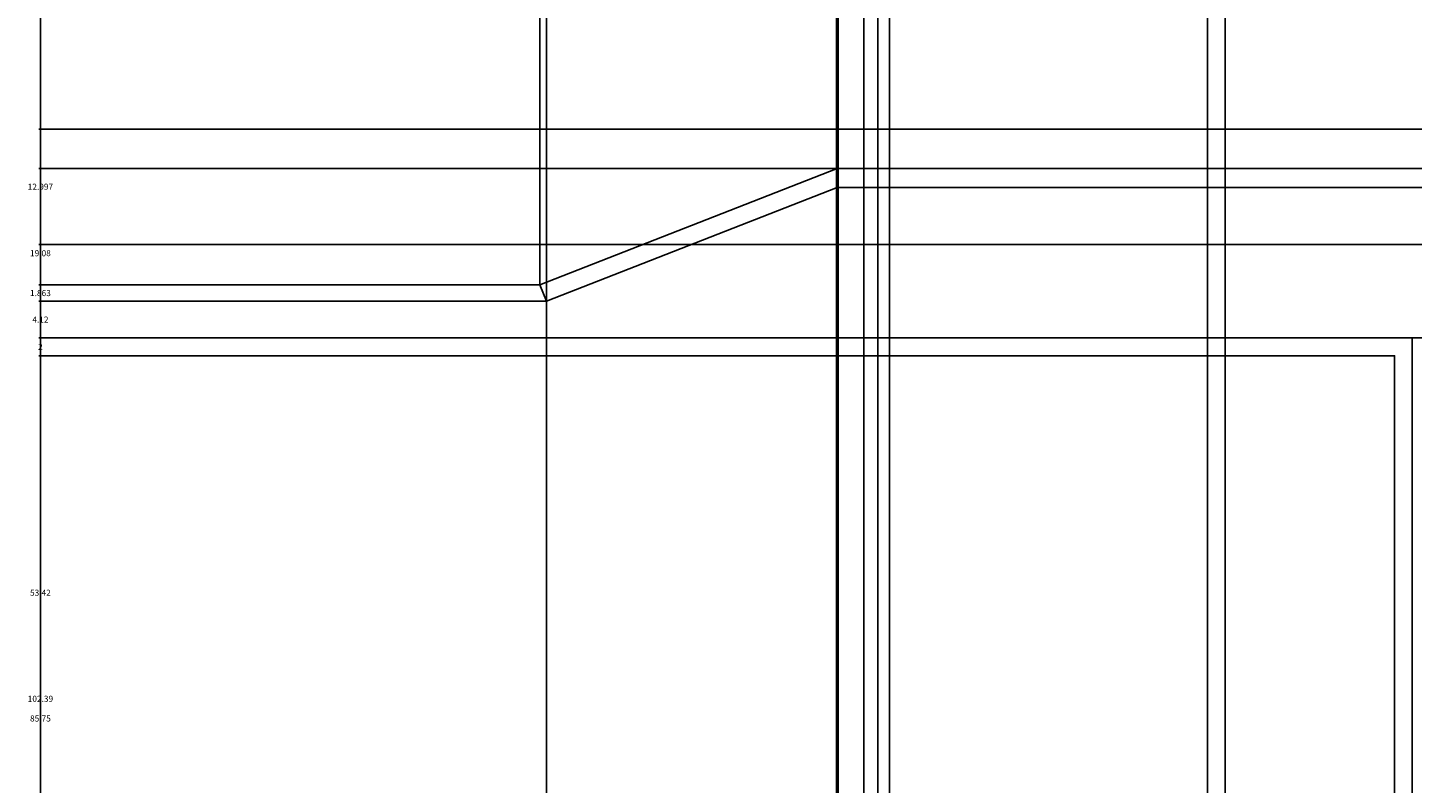
# Model space of a CAD drawing. Units: inches. Extents: x -139 to 346, y 72 to 413.
# Tile 2 of 18: x -139 to 18, y 157 to 242. Entities that reach past the tile are written whole.
import ezdxf

# ---------------------------------------------------------------- set-up
doc = ezdxf.new("R2010")
doc.units = ezdxf.units.IN
doc.header["$MEASUREMENT"] = 0
for name, color, linetype, lineweight in [('A-ANNO-DIMS', 2, 'Continuous', 18), ('A-ELEV', 9, 'Continuous', 25), ('A-GLAZ', 4, 'Continuous', 25), ('A-WALL', 7, 'Continuous', 50)]:
    doc.layers.add(name, color=color, linetype=linetype, lineweight=lineweight)
doc.styles.get("Standard").update_dxf_attribs({"font": 'arial.ttf'})
doc.dimstyles.get("Standard").update_dxf_attribs({"dimtxt": 0.6875, "dimasz": 0.18, "dimexe": 0.18, "dimexo": 0.0625, "dimgap": 0.09, "dimtad": 0, "dimtih": 1, "dimtoh": 1, "dimdec": 4, "dimzin": 0, "dimdsep": 46, "dimlunit": 4, "dimtxsty": 'Standard', "dimcen": 0.09, "dimadec": 0, "dimazin": 0, "dimtfac": 1, "dimtdec": 4, "dimtofl": 0, "dimtmove": 0, "dimatfit": 3, "dimfxl": 1, "dimtolj": 1, "dimtzin": 0, "dimarcsym": 0})

# ---------------------------------------------------------------- blocks, each defined once
blk = doc.blocks.new('*D41')
at = {"layer": 'A-ANNO-DIMS', "color": 0, "lineweight": -2, "transparency": 16777216}
for p, q in [((-47.34, 207.52), (-137.3, 207.52)), ((-137.12, 207.34), (-137.12, 165.09)), ((-137.12, 121.96), (-137.12, 164.21)), ((-5.6, 121.78), (-137.3, 121.78))]:
    blk.add_line(p, q, dxfattribs=at)
at = {"layer": 'A-ANNO-DIMS', "color": 0, "transparency": 16777216}
for points in [[(-137.15, 207.34), (-137.09, 207.34), (-137.12, 207.52)], [(-137.15, 121.96), (-137.09, 121.96), (-137.12, 121.78)]]:
    blk.add_solid(points, dxfattribs=at)
at = {"layer": 'Defpoints', "color": 0, "transparency": 16777216}
for p in [(-137.12, 207.52), (-47.27, 207.52), (-5.54, 121.78)]:
    blk.add_point(p, dxfattribs=at)
at = {"layer": 'A-ANNO-DIMS', "color": 0, "transparency": 16777216, "insert": (-137.12, 164.65), "char_height": 0.688, "attachment_point": 5}
blk.add_mtext('\\A1;85.75', dxfattribs=at)
blk = doc.blocks.new('*D42')
at = {"layer": 'A-ANNO-DIMS', "color": 0, "lineweight": -2, "transparency": 16777216}
for p, q in [((-47.34, 289.06), (-137.3, 289.06)), ((-137.12, 288.88), (-137.12, 248.73)), ((-137.12, 207.7), (-137.12, 247.85)), ((-47.34, 207.52), (-137.3, 207.52))]:
    blk.add_line(p, q, dxfattribs=at)
at = {"layer": 'A-ANNO-DIMS', "color": 0, "transparency": 16777216}
for points in [[(-137.15, 288.88), (-137.09, 288.88), (-137.12, 289.06)], [(-137.15, 207.7), (-137.09, 207.7), (-137.12, 207.52)]]:
    blk.add_solid(points, dxfattribs=at)
at = {"layer": 'Defpoints', "color": 0, "transparency": 16777216}
for p in [(-137.12, 289.06), (-47.27, 289.06), (-47.27, 207.52)]:
    blk.add_point(p, dxfattribs=at)
at = {"layer": 'A-ANNO-DIMS', "color": 0, "transparency": 16777216, "insert": (-137.12, 248.29), "char_height": 0.688, "attachment_point": 5}
blk.add_mtext('\\A1;81.54', dxfattribs=at)
blk = doc.blocks.new('*D48')
at = {"layer": 'A-ANNO-DIMS', "color": 0, "lineweight": -2, "transparency": 16777216}
for p, q in [((-47.34, 226.61), (-137.3, 226.61)), ((-137.12, 226.43), (-137.12, 217.51)), ((-137.12, 207.7), (-137.12, 216.62)), ((-47.34, 207.52), (-137.3, 207.52))]:
    blk.add_line(p, q, dxfattribs=at)
at = {"layer": 'A-ANNO-DIMS', "color": 0, "transparency": 16777216}
for points in [[(-137.15, 226.43), (-137.09, 226.43), (-137.12, 226.61)], [(-137.15, 207.7), (-137.09, 207.7), (-137.12, 207.52)]]:
    blk.add_solid(points, dxfattribs=at)
at = {"layer": 'Defpoints', "color": 0, "transparency": 16777216}
for p in [(-137.12, 226.61), (-47.27, 226.61), (-47.27, 207.52)]:
    blk.add_point(p, dxfattribs=at)
at = {"layer": 'A-ANNO-DIMS', "color": 0, "transparency": 16777216, "insert": (-137.12, 217.07), "char_height": 0.688, "attachment_point": 5}
blk.add_mtext('\\A1;19.08', dxfattribs=at)
blk = doc.blocks.new('*D49')
at = {"layer": 'A-ANNO-DIMS', "color": 0, "lineweight": -2, "transparency": 16777216}
for p, q in [((-80.8, 213.57), (-80.8, 412.45)), ((-80.62, 412.27), (-65.28, 412.27)), ((-47.45, 412.27), (-62.79, 412.27)), ((-47.27, 226.67), (-47.27, 412.45))]:
    blk.add_line(p, q, dxfattribs=at)
at = {"layer": 'A-ANNO-DIMS', "color": 0, "transparency": 16777216}
for points in [[(-80.62, 412.3), (-80.62, 412.24), (-80.8, 412.27)], [(-47.45, 412.3), (-47.45, 412.24), (-47.27, 412.27)]]:
    blk.add_solid(points, dxfattribs=at)
at = {"layer": 'Defpoints', "color": 0, "transparency": 16777216}
for p in [(-47.27, 412.27), (-47.27, 226.61), (-80.8, 213.51)]:
    blk.add_point(p, dxfattribs=at)
at = {"layer": 'A-ANNO-DIMS', "color": 0, "transparency": 16777216, "insert": (-64.03, 412.27), "char_height": 0.688, "attachment_point": 5}
blk.add_mtext('\\A1;33.52', dxfattribs=at)
blk = doc.blocks.new('*D50')
at = {"layer": 'A-ANNO-DIMS', "color": 0, "lineweight": -2, "transparency": 16777216}
for p, q in [((-80.8, 213.57), (-80.8, 412.45)), ((-80.62, 412.27), (-80.25, 412.27)), ((-80.07, 211.71), (-80.07, 412.45)), ((-80.07, 412.27), (-79.89, 412.27))]:
    blk.add_line(p, q, dxfattribs=at)
at = {"layer": 'A-ANNO-DIMS', "color": 0, "transparency": 16777216}
for points in [[(-80.62, 412.3), (-80.62, 412.24), (-80.8, 412.27)], [(-80.25, 412.3), (-80.25, 412.24), (-80.07, 412.27)]]:
    blk.add_solid(points, dxfattribs=at)
at = {"layer": 'Defpoints', "color": 0, "transparency": 16777216}
for p in [(-80.07, 412.27), (-80.8, 213.51), (-80.07, 211.65)]:
    blk.add_point(p, dxfattribs=at)
at = {"layer": 'A-ANNO-DIMS', "color": 0, "transparency": 16777216, "insert": (-78.91, 412.27), "char_height": 0.688, "attachment_point": 5}
blk.add_mtext('\\A1;0.73', dxfattribs=at)
blk = doc.blocks.new('*D51')
at = {"layer": 'A-ANNO-DIMS', "color": 0, "lineweight": -2, "transparency": 16777216}
for p, q in [((-80.07, 207.46), (-80.07, 72.49)), ((-47.27, 207.46), (-47.27, 72.49)), ((-79.89, 72.67), (-65.19, 72.67)), ((-47.45, 72.67), (-62.15, 72.67))]:
    blk.add_line(p, q, dxfattribs=at)
at = {"layer": 'A-ANNO-DIMS', "color": 0, "transparency": 16777216}
for points in [[(-79.89, 72.7), (-79.89, 72.64), (-80.07, 72.67)], [(-47.45, 72.7), (-47.45, 72.64), (-47.27, 72.67)]]:
    blk.add_solid(points, dxfattribs=at)
at = {"layer": 'Defpoints', "color": 0, "transparency": 16777216}
for p in [(-80.07, 207.52), (-47.27, 207.52), (-47.27, 72.67)]:
    blk.add_point(p, dxfattribs=at)
at = {"layer": 'A-ANNO-DIMS', "color": 0, "transparency": 16777216, "insert": (-63.67, 72.67), "char_height": 0.688, "attachment_point": 5}
blk.add_mtext('\\A1;32.795', dxfattribs=at)
blk = doc.blocks.new('*D52')
at = {"layer": 'A-ANNO-DIMS', "color": 0, "lineweight": -2, "transparency": 16777216}
for p, q in [((-80.13, 211.65), (-137.3, 211.65)), ((-137.12, 211.47), (-137.12, 210.02)), ((-137.12, 207.7), (-137.12, 209.15)), ((-80.13, 207.52), (-137.3, 207.52))]:
    blk.add_line(p, q, dxfattribs=at)
at = {"layer": 'A-ANNO-DIMS', "color": 0, "transparency": 16777216}
for points in [[(-137.15, 211.47), (-137.09, 211.47), (-137.12, 211.65)], [(-137.15, 207.7), (-137.09, 207.7), (-137.12, 207.52)]]:
    blk.add_solid(points, dxfattribs=at)
at = {"layer": 'Defpoints', "color": 0, "transparency": 16777216}
for p in [(-137.12, 211.65), (-80.07, 211.65), (-80.07, 207.52)]:
    blk.add_point(p, dxfattribs=at)
at = {"layer": 'A-ANNO-DIMS', "color": 0, "transparency": 16777216, "insert": (-137.12, 209.59), "char_height": 0.688, "attachment_point": 5}
blk.add_mtext('\\A1;4.12', dxfattribs=at)
blk = doc.blocks.new('*D53')
at = {"layer": 'A-ANNO-DIMS', "color": 0, "lineweight": -2, "transparency": 16777216}
for p, q in [((-80.86, 213.51), (-137.3, 213.51)), ((-137.12, 213.33), (-137.12, 213.02)), ((-80.13, 211.65), (-137.3, 211.65)), ((-137.12, 211.83), (-137.12, 212.14))]:
    blk.add_line(p, q, dxfattribs=at)
at = {"layer": 'A-ANNO-DIMS', "color": 0, "transparency": 16777216}
for points in [[(-137.15, 213.33), (-137.09, 213.33), (-137.12, 213.51)], [(-137.15, 211.83), (-137.09, 211.83), (-137.12, 211.65)]]:
    blk.add_solid(points, dxfattribs=at)
at = {"layer": 'Defpoints', "color": 0, "transparency": 16777216}
for p in [(-137.12, 213.51), (-80.8, 213.51), (-80.07, 211.65)]:
    blk.add_point(p, dxfattribs=at)
at = {"layer": 'A-ANNO-DIMS', "color": 0, "transparency": 16777216, "insert": (-137.12, 212.58), "char_height": 0.688, "attachment_point": 5}
blk.add_mtext('\\A1;1.863', dxfattribs=at)
blk = doc.blocks.new('*D54')
at = {"layer": 'A-ANNO-DIMS', "color": 0, "lineweight": -2, "transparency": 16777216}
for p, q in [((-47.21, 224.46), (344.39, 224.46)), ((344.21, 224.28), (344.21, 216.43)), ((344.21, 207.7), (344.21, 215.55)), ((-47.21, 207.52), (344.39, 207.52))]:
    blk.add_line(p, q, dxfattribs=at)
at = {"layer": 'A-ANNO-DIMS', "color": 0, "transparency": 16777216}
for points in [[(344.18, 224.28), (344.24, 224.28), (344.21, 224.46)], [(344.18, 207.7), (344.24, 207.7), (344.21, 207.52)]]:
    blk.add_solid(points, dxfattribs=at)
at = {"layer": 'Defpoints', "color": 0, "transparency": 16777216}
for p in [(-47.27, 224.46), (344.21, 224.46), (-47.27, 207.52)]:
    blk.add_point(p, dxfattribs=at)
at = {"layer": 'A-ANNO-DIMS', "color": 0, "transparency": 16777216, "insert": (344.21, 215.99), "char_height": 0.688, "attachment_point": 5}
blk.add_mtext('\\A1;16.935', dxfattribs=at)
blk = doc.blocks.new('*D55')
at = {"layer": 'A-ANNO-DIMS', "color": 0, "lineweight": -2, "transparency": 16777216}
for p, q in [((-47.21, 226.61), (344.39, 226.61)), ((344.21, 226.43), (344.21, 225.97)), ((344.21, 224.64), (344.21, 225.1)), ((-47.21, 224.46), (344.39, 224.46))]:
    blk.add_line(p, q, dxfattribs=at)
at = {"layer": 'A-ANNO-DIMS', "color": 0, "transparency": 16777216}
for points in [[(344.18, 226.43), (344.24, 226.43), (344.21, 226.61)], [(344.18, 224.64), (344.24, 224.64), (344.21, 224.46)]]:
    blk.add_solid(points, dxfattribs=at)
at = {"layer": 'Defpoints', "color": 0, "transparency": 16777216}
for p in [(-47.27, 226.61), (344.21, 226.61), (-47.27, 224.46)]:
    blk.add_point(p, dxfattribs=at)
at = {"layer": 'A-ANNO-DIMS', "color": 0, "transparency": 16777216, "insert": (344.21, 225.53), "char_height": 0.688, "attachment_point": 5}
blk.add_mtext('\\A1;2.147', dxfattribs=at)
blk = doc.blocks.new('*D59')
at = {"layer": 'A-ANNO-DIMS', "color": 0, "lineweight": -2, "transparency": 16777216}
for p, q in [((-3.6, 205.52), (-137.3, 205.52)), ((-137.12, 205.34), (-137.12, 179.26)), ((-137.12, 152.29), (-137.12, 178.37)), ((-3.6, 152.11), (-137.3, 152.11))]:
    blk.add_line(p, q, dxfattribs=at)
at = {"layer": 'A-ANNO-DIMS', "color": 0, "transparency": 16777216}
for points in [[(-137.15, 205.34), (-137.09, 205.34), (-137.12, 205.52)], [(-137.15, 152.29), (-137.09, 152.29), (-137.12, 152.11)]]:
    blk.add_solid(points, dxfattribs=at)
at = {"layer": 'Defpoints', "color": 0, "transparency": 16777216}
for p in [(-137.12, 205.52), (-3.54, 205.52), (-3.54, 152.11)]:
    blk.add_point(p, dxfattribs=at)
at = {"layer": 'A-ANNO-DIMS', "color": 0, "transparency": 16777216, "insert": (-137.12, 178.82), "char_height": 0.688, "attachment_point": 5}
blk.add_mtext('\\A1;53.42', dxfattribs=at)
blk = doc.blocks.new('*D60')
at = {"layer": 'A-ANNO-DIMS', "color": 0, "lineweight": -2, "transparency": 16777216}
for p, q in [((-5.6, 207.52), (-137.3, 207.52)), ((-137.12, 207.34), (-137.12, 206.96)), ((-137.12, 205.7), (-137.12, 206.09)), ((-3.6, 205.52), (-137.3, 205.52))]:
    blk.add_line(p, q, dxfattribs=at)
at = {"layer": 'A-ANNO-DIMS', "color": 0, "transparency": 16777216}
for points in [[(-137.15, 207.34), (-137.09, 207.34), (-137.12, 207.52)], [(-137.15, 205.7), (-137.09, 205.7), (-137.12, 205.52)]]:
    blk.add_solid(points, dxfattribs=at)
at = {"layer": 'Defpoints', "color": 0, "transparency": 16777216}
for p in [(-137.12, 207.52), (-5.54, 207.52), (-3.54, 205.52)]:
    blk.add_point(p, dxfattribs=at)
at = {"layer": 'A-ANNO-DIMS', "color": 0, "transparency": 16777216, "insert": (-137.12, 206.52), "char_height": 0.688, "attachment_point": 5}
blk.add_mtext('\\A1;2', dxfattribs=at)
blk = doc.blocks.new('*D61')
at = {"layer": 'A-ANNO-DIMS', "color": 0, "lineweight": -2, "transparency": 16777216}
for p, q in [((-5.6, 207.52), (-137.3, 207.52)), ((-137.12, 207.34), (-137.12, 165.09)), ((-137.12, 121.96), (-137.12, 164.21)), ((-5.6, 121.78), (-137.3, 121.78))]:
    blk.add_line(p, q, dxfattribs=at)
at = {"layer": 'A-ANNO-DIMS', "color": 0, "transparency": 16777216}
for points in [[(-137.15, 207.34), (-137.09, 207.34), (-137.12, 207.52)], [(-137.15, 121.96), (-137.09, 121.96), (-137.12, 121.78)]]:
    blk.add_solid(points, dxfattribs=at)
at = {"layer": 'Defpoints', "color": 0, "transparency": 16777216}
for p in [(-137.12, 207.52), (-5.54, 207.52), (-5.54, 121.78)]:
    blk.add_point(p, dxfattribs=at)
at = {"layer": 'A-ANNO-DIMS', "color": 0, "transparency": 16777216, "insert": (-137.12, 164.65), "char_height": 0.688, "attachment_point": 5}
blk.add_mtext('\\A1;85.75', dxfattribs=at)
blk = doc.blocks.new('*D68')
at = {"layer": 'A-ANNO-DIMS', "color": 0, "lineweight": -2, "transparency": 16777216}
for p, q in [((-5.54, 207.59), (-5.54, 412.45)), ((-5.36, 412.27), (-4.86, 412.27)), ((-3.72, 412.27), (-4.22, 412.27)), ((-3.54, 205.59), (-3.54, 412.45))]:
    blk.add_line(p, q, dxfattribs=at)
at = {"layer": 'A-ANNO-DIMS', "color": 0, "transparency": 16777216}
for points in [[(-5.36, 412.3), (-5.36, 412.24), (-5.54, 412.27)], [(-3.72, 412.3), (-3.72, 412.24), (-3.54, 412.27)]]:
    blk.add_solid(points, dxfattribs=at)
at = {"layer": 'Defpoints', "color": 0, "transparency": 16777216}
for p in [(-3.54, 412.27), (-5.54, 207.52), (-3.54, 205.52)]:
    blk.add_point(p, dxfattribs=at)
at = {"layer": 'A-ANNO-DIMS', "color": 0, "transparency": 16777216, "insert": (-4.54, 412.27), "char_height": 0.688, "attachment_point": 5}
blk.add_mtext('\\A1;2', dxfattribs=at)
blk = doc.blocks.new('*D70')
at = {"layer": 'A-ANNO-DIMS', "color": 0, "lineweight": -2, "transparency": 16777216}
for p, q in [((125.18, 218.06), (-137.3, 218.06)), ((-137.12, 217.88), (-137.12, 167.31)), ((-137.12, 115.86), (-137.12, 166.43)), ((125.18, 115.68), (-137.3, 115.68))]:
    blk.add_line(p, q, dxfattribs=at)
at = {"layer": 'A-ANNO-DIMS', "color": 0, "transparency": 16777216}
for points in [[(-137.15, 217.88), (-137.09, 217.88), (-137.12, 218.06)], [(-137.15, 115.86), (-137.09, 115.86), (-137.12, 115.68)]]:
    blk.add_solid(points, dxfattribs=at)
at = {"layer": 'Defpoints', "color": 0, "transparency": 16777216}
for p in [(-137.12, 218.06), (125.25, 218.06), (125.25, 115.68)]:
    blk.add_point(p, dxfattribs=at)
at = {"layer": 'A-ANNO-DIMS', "color": 0, "transparency": 16777216, "insert": (-137.12, 166.87), "char_height": 0.688, "attachment_point": 5}
blk.add_mtext('\\A1;102.39', dxfattribs=at)
blk = doc.blocks.new('*D71')
at = {"layer": 'A-ANNO-DIMS', "color": 0, "lineweight": -2, "transparency": 16777216}
for p, q in [((120.44, 231.06), (-137.3, 231.06)), ((-137.12, 230.88), (-137.12, 225)), ((-137.12, 218.24), (-137.12, 224.12)), ((125.18, 218.06), (-137.3, 218.06))]:
    blk.add_line(p, q, dxfattribs=at)
at = {"layer": 'A-ANNO-DIMS', "color": 0, "transparency": 16777216}
for points in [[(-137.15, 230.88), (-137.09, 230.88), (-137.12, 231.06)], [(-137.15, 218.24), (-137.09, 218.24), (-137.12, 218.06)]]:
    blk.add_solid(points, dxfattribs=at)
at = {"layer": 'Defpoints', "color": 0, "transparency": 16777216}
for p in [(-137.12, 231.06), (120.51, 231.06), (125.25, 218.06)]:
    blk.add_point(p, dxfattribs=at)
at = {"layer": 'A-ANNO-DIMS', "color": 0, "transparency": 16777216, "insert": (-137.12, 224.56), "char_height": 0.688, "attachment_point": 5}
blk.add_mtext('\\A1;12.997', dxfattribs=at)
blk = doc.blocks.new('*D93')
at = {"layer": 'A-ANNO-DIMS', "color": 0, "lineweight": -2, "transparency": 16777216}
for p, q in [((-44.29, 298.23), (-44.29, 72.49)), ((-42.71, 291), (-42.71, 72.49)), ((-44.11, 72.67), (-42.89, 72.67)), ((-42.71, 72.67), (-42.53, 72.67))]:
    blk.add_line(p, q, dxfattribs=at)
at = {"layer": 'A-ANNO-DIMS', "color": 0, "transparency": 16777216}
for points in [[(-44.11, 72.7), (-44.11, 72.64), (-44.29, 72.67)], [(-42.89, 72.7), (-42.89, 72.64), (-42.71, 72.67)]]:
    blk.add_solid(points, dxfattribs=at)
at = {"layer": 'Defpoints', "color": 0, "transparency": 16777216}
for p in [(-44.29, 298.29), (-42.71, 291.06), (-42.71, 72.67)]:
    blk.add_point(p, dxfattribs=at)
at = {"layer": 'A-ANNO-DIMS', "color": 0, "transparency": 16777216, "insert": (-41.58, 72.67), "char_height": 0.688, "attachment_point": 5}
blk.add_mtext('\\A1;1.58', dxfattribs=at)
blk = doc.blocks.new('*D94')
at = {"layer": 'A-ANNO-DIMS', "color": 0, "lineweight": -2, "transparency": 16777216}
for p, q in [((-42.71, 291), (-42.71, 72.49)), ((-41.4, 291), (-41.4, 72.49)), ((-42.53, 72.67), (-41.58, 72.67)), ((-41.4, 72.67), (-41.22, 72.67))]:
    blk.add_line(p, q, dxfattribs=at)
at = {"layer": 'A-ANNO-DIMS', "color": 0, "transparency": 16777216}
for points in [[(-42.53, 72.7), (-42.53, 72.64), (-42.71, 72.67)], [(-41.58, 72.7), (-41.58, 72.64), (-41.4, 72.67)]]:
    blk.add_solid(points, dxfattribs=at)
at = {"layer": 'Defpoints', "color": 0, "transparency": 16777216}
for p in [(-42.71, 291.06), (-41.4, 291.06), (-41.4, 72.67)]:
    blk.add_point(p, dxfattribs=at)
at = {"layer": 'A-ANNO-DIMS', "color": 0, "transparency": 16777216, "insert": (-40.27, 72.67), "char_height": 0.688, "attachment_point": 5}
blk.add_mtext('\\A1;1.32', dxfattribs=at)

msp = doc.modelspace()

# ---------------------------------------------------------------- linework, layer by layer
at = {"layer": 'A-ELEV'}
for p, q in [((-80.7961, 213.5107), (-47.2734, 226.6062)), ((-80.0684, 211.6478), (-47.2734, 224.4591)), ((-80.0684, 211.6478), (-80.7961, 213.5107)), ((-80.0684, 207.5243), (-80.0684, 211.6478)), ((-47.2734, 207.5243), (-80.0684, 207.5243))]:
    msp.add_line(p, q, dxfattribs=at)
at = {"layer": 'A-GLAZ'}
for points in [[(-5.5402, 207.5243), (17.5525, 207.5243), (17.5525, 121.7753), (-5.5402, 121.7753)], [(-3.5402, 205.5243), (15.5525, 205.5243), (15.5525, 123.7753), (-3.5402, 123.7753)]]:
    msp.add_lwpolyline(points, close=True, dxfattribs=at)
at = {"layer": 'A-WALL'}
msp.add_line((-47.2734, 291.0604), (-47.2734, 94.9748), dxfattribs=at)

# ---------------------------------------------------------------- dimensions: what is measured, and where the dimension line sits
at = {"layer": 'A-ANNO-DIMS'}
for base, p1, p2, override, picture, middle in [((-47.2734, 412.2748), (-80.7961, 213.5107), (-47.2734, 226.6062), {"dimdec": 2, "dimlfac": 1, "dimrnd": 0, "dimzin": 0, "dimdsep": 46, "dimlunit": 2}, '*D49', (-64.0348, 412.2748)), ((-80.0684, 412.2748), (-80.7961, 213.5107), (-80.0684, 211.6478), {"dimdec": 2, "dimlfac": 1, "dimrnd": 0, "dimzin": 0, "dimdsep": 46, "dimlunit": 2}, '*D50', (-78.9055, 412.2748)), ((-3.5402, 412.2748), (-5.5402, 207.5243), (-3.5402, 205.5243), {"dimdec": 0, "dimlfac": 1, "dimrnd": 0, "dimzin": 0, "dimdsep": 46, "dimlunit": 2}, '*D68', (-4.5402, 412.2748)), ((-42.7149, 72.6748), (-44.2923, 298.293), (-42.7149, 291.0604), {"dimdec": 2, "dimlfac": 1, "dimrnd": 0, "dimzin": 0, "dimdsep": 46, "dimlunit": 2}, '*D93', (-41.5836, 72.6748)), ((-41.3972, 72.6748), (-42.7149, 291.0604), (-41.3972, 291.0604), {"dimdec": 2, "dimlfac": 1, "dimrnd": 0, "dimzin": 0, "dimdsep": 46, "dimlunit": 2}, '*D94', (-40.2702, 72.6748)), ((-47.2734, 72.6748), (-80.0684, 207.5243), (-47.2734, 207.5243), {"dimdec": 3, "dimlfac": 1, "dimrnd": 0, "dimzin": 0, "dimdsep": 46, "dimlunit": 2}, '*D51', (-63.6709, 72.6748))]:
    dim = msp.add_linear_dim(base=base, p1=p1, p2=p2, dimstyle='Standard', override=override, dxfattribs=at)
    dim.commit()
    dim.dimension.update_dxf_attribs({"geometry": picture, "text_midpoint": middle})
for base, p1, p2, override, picture, middle in [((-137.1237, 289.0604), (-47.2734, 207.5243), (-47.2734, 289.0604), {"dimdec": 2, "dimlfac": 1, "dimrnd": 0, "dimzin": 0, "dimdsep": 46, "dimlunit": 2}, '*D42', (-137.1237, 248.2924)), ((-137.1237, 231.0607), (125.2464, 218.0635), (120.5054, 231.0607), {"dimdec": 3, "dimlfac": 1, "dimrnd": 0, "dimzin": 0, "dimdsep": 46, "dimlunit": 2}, '*D71', (-137.1237, 224.5621)), ((-137.1237, 226.6062), (-47.2734, 207.5243), (-47.2734, 226.6062), {"dimdec": 2, "dimlfac": 1, "dimrnd": 0, "dimzin": 0, "dimdsep": 46, "dimlunit": 2}, '*D48', (-137.1237, 217.0653)), ((344.2055, 226.6062), (-47.2734, 224.4591), (-47.2734, 226.6062), {"dimdec": 3, "dimlfac": 1, "dimrnd": 0, "dimzin": 0, "dimdsep": 46, "dimlunit": 2}, '*D55', (344.2055, 225.5327)), ((344.2055, 224.4591), (-47.2734, 207.5243), (-47.2734, 224.4591), {"dimdec": 3, "dimlfac": 1, "dimrnd": 0, "dimzin": 0, "dimdsep": 46, "dimlunit": 2}, '*D54', (344.2055, 215.9917)), ((-137.1237, 218.0635), (125.2464, 115.6761), (125.2464, 218.0635), {"dimdec": 2, "dimlfac": 1, "dimrnd": 0, "dimzin": 0, "dimdsep": 46, "dimlunit": 2}, '*D70', (-137.1237, 166.8698)), ((-137.1237, 213.5107), (-80.0684, 211.6478), (-80.7961, 213.5107), {"dimdec": 3, "dimlfac": 1, "dimrnd": 0, "dimzin": 0, "dimdsep": 46, "dimlunit": 2}, '*D53', (-137.1237, 212.5793)), ((-137.1237, 211.6478), (-80.0684, 207.5243), (-80.0684, 211.6478), {"dimdec": 2, "dimlfac": 1, "dimrnd": 0, "dimzin": 0, "dimdsep": 46, "dimlunit": 2}, '*D52', (-137.1237, 209.5861)), ((-137.1237, 207.5243), (-5.5402, 121.7753), (-47.2734, 207.5243), {"dimdec": 2, "dimlfac": 1, "dimrnd": 0, "dimzin": 0, "dimdsep": 46, "dimlunit": 2}, '*D41', (-137.1237, 164.6498)), ((-137.1237, 207.5243), (-5.5402, 121.7753), (-5.5402, 207.5243), {"dimdec": 2, "dimlfac": 1, "dimrnd": 0, "dimzin": 0, "dimdsep": 46, "dimlunit": 2}, '*D61', (-137.1237, 164.6498)), ((-137.1237, 207.5243), (-3.5402, 205.5243), (-5.5402, 207.5243), {"dimdec": 0, "dimlfac": 1, "dimrnd": 0, "dimzin": 0, "dimdsep": 46, "dimlunit": 2}, '*D60', (-137.1237, 206.5243)), ((-137.1237, 205.5243), (-3.5402, 152.1076), (-3.5402, 205.5243), {"dimdec": 2, "dimlfac": 1, "dimrnd": 0, "dimzin": 0, "dimdsep": 46, "dimlunit": 2}, '*D59', (-137.1237, 178.8159))]:
    dim = msp.add_linear_dim(base=base, p1=p1, p2=p2, angle=90, dimstyle='Standard', override=override, dxfattribs=at)
    dim.commit()
    dim.dimension.update_dxf_attribs({"geometry": picture, "text_midpoint": middle})

doc.saveas('drawing.dxf')
